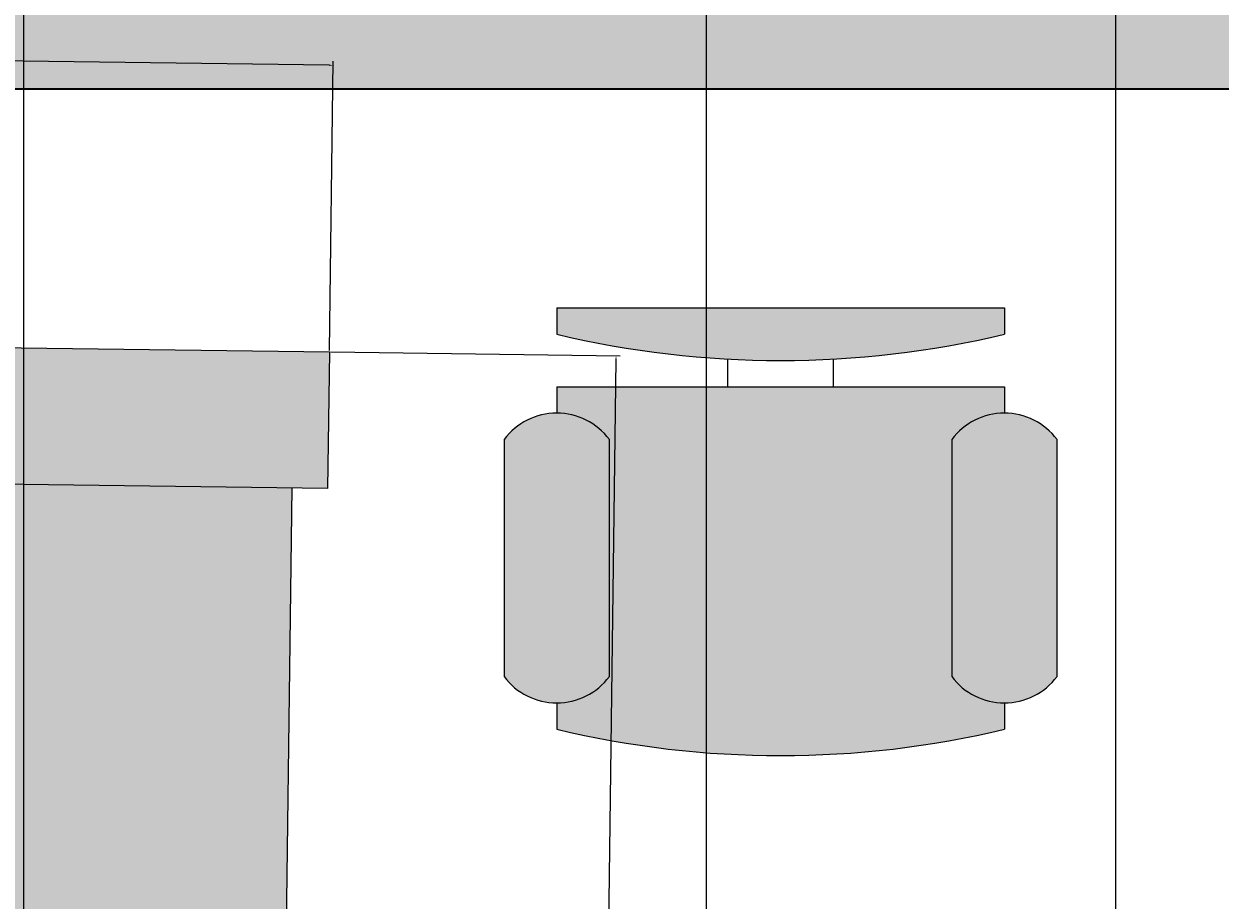
# Model space of a CAD drawing. Units: inches. Extents: x 1567 to 1964, y 1813 to 2447.
# Tile 10 of 28: x 1630 to 1683, y 2224 to 2262. Entities that reach past the tile are written whole.
import ezdxf

# ---------------------------------------------------------------- set-up
doc = ezdxf.new("R2010")
doc.units = ezdxf.units.IN
for name, color, linetype, lineweight in [('A-ANNO-DIMS', 2, 'Continuous', 18), ('A-FURN', 8, 'Continuous', 18), ('A-WALL', 7, 'Continuous', 35)]:
    doc.layers.add(name, color=color, linetype=linetype, lineweight=lineweight)
doc.layers.add('A-FURN-PATT', color=252, linetype='Continuous', lineweight=13, true_color=0x939598)
doc.layers.add('A-WALL-PATT', color=251, linetype='Continuous', lineweight=13, true_color=0x636466)
doc.styles.get("Standard").update_dxf_attribs({"font": 'arial.ttf'})
doc.dimstyles.get("Standard").update_dxf_attribs({"dimtxt": 0.18, "dimasz": 0.18, "dimexe": 0.18, "dimexo": 0.0625, "dimgap": 0.09, "dimtad": 0, "dimtih": 1, "dimtoh": 1, "dimdec": 4, "dimzin": 0, "dimdsep": 46, "dimtxsty": 'Standard', "dimcen": 0.09, "dimadec": 0, "dimazin": 0, "dimtfac": 1, "dimtdec": 4, "dimtofl": 0, "dimtmove": 0, "dimatfit": 3, "dimfxl": 1, "dimtolj": 1, "dimtzin": 0, "dimarcsym": 0})

# ---------------------------------------------------------------- blocks, each defined once
blk = doc.blocks.new('Sofa - Roundback 7 ft.')
for p, q in [((35.99998, -34), (35.99998, -11.4696)), ((-36.000027, -32.4421), (35.99998, -32.4421))]:
    blk.add_line(p, q)
blk.add_lwpolyline([(41.99998, -8), (41.99998, -34), (35.99998, -34)])
blk = doc.blocks.new('Chair - Desk')
for p, q in [((-8.5, 0), (-8.5, -1)), ((-8.5, 0), (8.5, 0)), ((8.5, 0), (8.5, -1)), ((-2, -3), (-2, -1.9355)), ((2, -1.9576), (2, -3)), ((-8.5, -3), (-8.5, -4)), ((-8.5, -3), (8.5, -3)), ((8.5, -3), (8.5, -4)), ((-10.5, -5), (-10.5, -14)), ((-6.5, -14), (-6.5, -5)), ((6.5, -5), (6.5, -14)), ((10.5, -14), (10.5, -5)), ((-8.5, -15), (-8.5, -16)), ((8.5, -15), (8.5, -16))]:
    blk.add_line(p, q)
for centre, radius, start, end in [((0, 34.625), 36.625, 256.5803, 283.4197), ((-8.5, -6.5), 2.5, 36.8699, 143.1301), ((8.5, -6.5), 2.5, 36.8699, 143.1301), ((-8.5, -12.5), 2.5, 216.8699, 323.1301), ((8.5, -12.5), 2.5, 216.8699, 323.1301), ((0, 19.625), 36.625, 256.5803, 283.4197)]:
    blk.add_arc(centre, radius, start, end)
blk = doc.blocks.new('*D23')
at = {"layer": 'A-ANNO-DIMS', "color": 0, "lineweight": -2, "transparency": 16777216}
for p, q in [((1643.923, 2247.723), (1656.64, 2247.554)), ((1656.457, 2247.376), (1655.905, 2205.743)), ((1655.347, 2163.744), (1655.9, 2205.377)), ((1642.808, 2163.73), (1655.525, 2163.561))]:
    blk.add_line(p, q, dxfattribs=at)
at = {"layer": 'A-ANNO-DIMS', "color": 0, "transparency": 16777216}
for points in [[(1656.427, 2247.377), (1656.487, 2247.376), (1656.46, 2247.556)], [(1655.317, 2163.744), (1655.377, 2163.743), (1655.345, 2163.564)]]:
    blk.add_solid(points, dxfattribs=at)
at = {"layer": 'Defpoints', "color": 0, "transparency": 16777216}
for p in [(1643.861, 2247.723), (1656.46, 2247.556), (1642.746, 2163.731)]:
    blk.add_point(p, dxfattribs=at)
at = {"layer": 'A-ANNO-DIMS', "color": 0, "transparency": 16777216, "insert": (1655.902, 2205.56), "char_height": 0.18, "attachment_point": 5}
blk.add_mtext('\\A1;SOFA 84', dxfattribs=at)
blk = doc.blocks.new('*D24')
at = {"layer": 'A-ANNO-DIMS', "color": 0, "lineweight": -2, "transparency": 16777216}
for p, q in [((1607.198, 2248.273), (1607.367, 2260.989)), ((1607.544, 2260.807), (1625.477, 2260.569)), ((1643.848, 2260.325), (1625.915, 2260.563)), ((1643.862, 2247.786), (1644.03, 2260.502))]:
    blk.add_line(p, q, dxfattribs=at)
at = {"layer": 'A-ANNO-DIMS', "color": 0, "transparency": 16777216}
for points in [[(1607.545, 2260.837), (1607.544, 2260.777), (1607.364, 2260.809)], [(1643.848, 2260.355), (1643.848, 2260.295), (1644.028, 2260.322)]]:
    blk.add_solid(points, dxfattribs=at)
at = {"layer": 'Defpoints', "color": 0, "transparency": 16777216}
for p in [(1607.364, 2260.809), (1607.197, 2248.21), (1643.861, 2247.723)]:
    blk.add_point(p, dxfattribs=at)
at = {"layer": 'A-ANNO-DIMS', "color": 0, "transparency": 16777216, "insert": (1625.696, 2260.566), "char_height": 0.18, "attachment_point": 5}
blk.add_mtext('\\A1;37', dxfattribs=at)
blk = doc.blocks.new('*D57')
at = {"layer": 'A-ANNO-DIMS', "color": 0, "lineweight": -2, "transparency": 16777216}
for p, q in [((1630.43, 2127.352), (1630.43, 2447.12)), ((1630.61, 2446.94), (1654.207, 2446.94)), ((1678.25, 2446.94), (1654.652, 2446.94)), ((1678.43, 2127.352), (1678.43, 2447.12))]:
    blk.add_line(p, q, dxfattribs=at)
at = {"layer": 'A-ANNO-DIMS', "color": 0, "transparency": 16777216}
for points in [[(1630.61, 2446.97), (1630.61, 2446.91), (1630.43, 2446.94)], [(1678.25, 2446.97), (1678.25, 2446.91), (1678.43, 2446.94)]]:
    blk.add_solid(points, dxfattribs=at)
at = {"layer": 'Defpoints', "color": 0, "transparency": 16777216}
for p in [(1678.43, 2446.94), (1630.43, 2127.29), (1678.43, 2127.29)]:
    blk.add_point(p, dxfattribs=at)
at = {"layer": 'A-ANNO-DIMS', "color": 0, "transparency": 16777216, "insert": (1654.43, 2446.94), "char_height": 0.18, "attachment_point": 5}
blk.add_mtext('\\A1;48', dxfattribs=at)
blk = doc.blocks.new('*D60')
at = {"layer": 'A-ANNO-DIMS', "color": 0, "lineweight": -2, "transparency": 16777216}
for p, q in [((1660.43, 2063.352), (1660.43, 2447.12)), ((1660.61, 2446.94), (1681.208, 2446.94)), ((1702.25, 2446.94), (1681.651, 2446.94)), ((1702.43, 2063.352), (1702.43, 2447.12))]:
    blk.add_line(p, q, dxfattribs=at)
at = {"layer": 'A-ANNO-DIMS', "color": 0, "transparency": 16777216}
for points in [[(1660.61, 2446.97), (1660.61, 2446.91), (1660.43, 2446.94)], [(1702.25, 2446.97), (1702.25, 2446.91), (1702.43, 2446.94)]]:
    blk.add_solid(points, dxfattribs=at)
at = {"layer": 'Defpoints', "color": 0, "transparency": 16777216}
for p in [(1660.43, 2446.94), (1660.43, 2063.29), (1702.43, 2063.29)]:
    blk.add_point(p, dxfattribs=at)
at = {"layer": 'A-ANNO-DIMS', "color": 0, "transparency": 16777216, "insert": (1681.43, 2446.94), "char_height": 0.18, "attachment_point": 5}
blk.add_mtext('\\A1;42', dxfattribs=at)

msp = doc.modelspace()

# ---------------------------------------------------------------- hatches: boundary and pattern name
at = {"layer": 'A-FURN-PATT'}
h = msp.add_hatch(color=256, dxfattribs=at)
h.dxf.hatch_style = 1
h.paths.add_polyline_path([(1621.2532, 2242.0229), (1643.7811, 2241.7239), (1643.8607, 2247.7234), (1617.863, 2248.0685, 0.1904762), (1616.7481, 2164.0759), (1642.7458, 2163.7308), (1642.8254, 2169.7302), (1620.2975, 2170.0293, -0.1519478)])
h.paths.add_polyline_path([(1673.5306, 2249.6607), (1653.8509, 2249.6607), (1653.8509, 2248.5031, 0.1176471), (1673.5306, 2248.5031)])
h.paths.add_polyline_path([(1706.0889, 2249.6607), (1686.4092, 2249.6607), (1686.4092, 2248.5031, 0.1176471), (1706.0889, 2248.5031)])
h.paths.add_polyline_path([(1782.4511, 2227.4197), (1766.4511, 2227.4197), (1766.2949, 2226.4197), (1782.6074, 2226.4197)])
h.paths.add_polyline_path([(1810.4511, 2227.4197), (1794.4511, 2227.4197), (1794.2949, 2226.4197), (1810.6074, 2226.4197)])
h.paths.add_polyline_path([(1743.9511, 2208.076), (1742.9511, 2207.9197), (1742.9511, 2191.9197), (1743.9511, 2191.7635)])
h.paths.add_polyline_path([(1782.6074, 2173.4197), (1766.2949, 2173.4197), (1766.4511, 2172.4197), (1782.4511, 2172.4197)])
h.paths.add_polyline_path([(1810.6074, 2173.4197), (1794.2949, 2173.4197), (1794.4511, 2172.4197), (1810.4511, 2172.4197)])
h.paths.add_polyline_path([(1861.053, 2006.5071), (1845.8531, 2006.5071), (1861.053, 1991.3071)])
h.paths.add_polyline_path([(1905.853, 1993.7071), (1861.053, 1993.7071), (1861.053, 1991.3071), (1905.853, 1991.3071)])
h.paths.add_polyline_path([(1919.7245, 2257.29, 0.5000001), (1918.7245, 2258.29), (1901.7245, 2258.29, 0.5000001), (1900.7245, 2257.29), (1900.7245, 2253.29, 0.5000001), (1901.7245, 2252.29), (1918.7245, 2252.29, 0.5000001), (1919.7245, 2253.29)])
h.paths.add_polyline_path([(1875.9094, 2391.0204), (1875.9094, 2375.8204), (1891.1093, 2375.8204)], flags=17)
h.paths.add_polyline_path([(1891.1093, 2405.4204), (1831.1094, 2405.4204), (1831.1094, 2391.0204), (1839.1093, 2391.0204), (1839.1093, 2404.2204), (1859.9093, 2404.2204), (1859.9093, 2391.0204), (1862.3093, 2391.0204), (1862.3093, 2404.2204), (1883.1093, 2404.2204), (1883.1093, 2389.0204), (1877.9094, 2389.0204), (1891.1093, 2375.8204)])
h.paths.add_polyline_path([(1682.1402, 2390.0316), (1682.1402, 2374.8316), (1697.3402, 2374.8316)], flags=17)
h.paths.add_polyline_path([(1697.3402, 2404.4316), (1637.3402, 2404.4316), (1637.3402, 2390.0316), (1645.3402, 2390.0316), (1645.3402, 2403.2316), (1666.1402, 2403.2316), (1666.1402, 2390.0316), (1668.5402, 2390.0316), (1668.5402, 2403.2316), (1689.3402, 2403.2316), (1689.3402, 2388.0316), (1684.1402, 2388.0316), (1697.3402, 2374.8316)])
h = msp.add_hatch(color=256, dxfattribs=at)
h.dxf.hatch_style = 1
h.paths.add_polyline_path([(1642.2233, 2241.7446), (1623.1648, 2241.9976), (1622.8462, 2217.9997), (1641.9047, 2217.7467)])
h.paths.add_polyline_path([(1641.9047, 2217.7467), (1622.8462, 2217.9997), (1622.5277, 2194.0018), (1641.5862, 2193.7488)])
h.paths.add_polyline_path([(1641.5862, 2193.7488), (1622.5277, 2194.0018), (1622.2091, 2170.0039), (1641.2677, 2169.7509)])
h.paths.add_polyline_path([(1671.2154, 2243.8726, -0.236068), (1673.5306, 2245.0302), (1673.5306, 2246.1879), (1653.8509, 2246.1879), (1653.8509, 2245.0302, -0.236068), (1656.1662, 2243.8726), (1656.1662, 2233.4539, -0.236068), (1653.8509, 2232.2963), (1653.8509, 2231.1387, 0.1176471), (1673.5306, 2231.1387), (1673.5306, 2232.2963, -0.236068), (1671.2154, 2233.4539)])
h.paths.add_polyline_path([(1703.7736, 2243.8726, -0.236068), (1706.0889, 2245.0302), (1706.0889, 2246.1879), (1686.4092, 2246.1879), (1686.4092, 2245.0302, -0.236068), (1688.7245, 2243.8726), (1688.7245, 2233.4539, -0.236068), (1686.4092, 2232.2963), (1686.4092, 2231.1387, 0.1176471), (1706.0889, 2231.1387), (1706.0889, 2232.2963, -0.236068), (1703.7736, 2233.4539)])
h.paths.add_polyline_path([(1782.6855, 2225.9197), (1766.2168, 2225.9197), (1764.9668, 2217.9197), (1783.9356, 2217.9197)])
h.paths.add_polyline_path([(1810.6855, 2225.9197), (1794.2168, 2225.9197), (1792.9668, 2217.9197), (1811.9356, 2217.9197)])
h.paths.add_polyline_path([(1752.4511, 2209.4041), (1744.4511, 2208.1541), (1744.4511, 2191.6853), (1752.4511, 2190.4354)])
h.paths.add_polyline_path([(1783.9356, 2181.9197), (1764.9668, 2181.9197), (1766.2168, 2173.9197), (1782.6855, 2173.9197)])
h.paths.add_polyline_path([(1811.9356, 2181.9197), (1792.9668, 2181.9197), (1794.2168, 2173.9197), (1810.6855, 2173.9197)])
h.paths.add_polyline_path([(1832.4511, 2208.1541), (1824.4511, 2209.4041), (1824.4511, 2190.4354), (1832.4511, 2191.6853)])
h.paths.add_polyline_path([(1824.4511, 2194.4197), (1823.8775, 2194.266), (1823.2838, 2194.1743), (1822.6735, 2194.1363), (1822.0501, 2194.1437), (1821.4169, 2194.1882), (1820.7773, 2194.2615), (1820.1348, 2194.3554), (1819.4928, 2194.4614), (1818.8527, 2194.5726), (1818.2083, 2194.6873), (1817.5511, 2194.8049), (1816.873, 2194.9249), (1816.1656, 2195.0469), (1815.4205, 2195.1704), (1814.6296, 2195.2948), (1813.7845, 2195.4197), (1812.88, 2195.5442), (1811.9238, 2195.6658), (1810.9265, 2195.7815), (1809.899, 2195.8885), (1808.852, 2195.9837), (1807.7962, 2196.0643), (1806.7423, 2196.1273), (1805.7011, 2196.1697), (1804.6806, 2196.1896), (1803.6777, 2196.188), (1802.6865, 2196.1668), (1801.7011, 2196.1281), (1800.7158, 2196.0737), (1799.7245, 2196.0057), (1798.7216, 2195.9259), (1797.7011, 2195.8364), (1796.6564, 2195.7387), (1795.5781, 2195.6333), (1794.4557, 2195.52), (1793.2792, 2195.3989), (1792.0383, 2195.27), (1790.7226, 2195.1333), (1789.3219, 2194.9887), (1787.8261, 2194.8364), (1786.1882, 2194.6764), (1784.2148, 2194.5096), (1781.6759, 2194.3369), (1778.3417, 2194.1593), (1773.9821, 2193.9778), (1768.3671, 2193.7934), (1761.2668, 2193.6071), (1752.4511, 2193.4197), (1752.4511, 2189.9197), (1762.0489, 2190.1067), (1769.9836, 2190.2908), (1776.4672, 2190.469), (1781.7115, 2190.6385), (1785.9285, 2190.7962), (1789.33, 2190.9393), (1792.128, 2191.0648), (1794.5344, 2191.1697), (1796.7278, 2191.2521), (1798.7532, 2191.313), (1800.6223, 2191.3543), (1802.3469, 2191.3781), (1803.9387, 2191.3862), (1805.4094, 2191.3807), (1806.7708, 2191.3634), (1808.0345, 2191.3364), (1809.2127, 2191.3013), (1810.3196, 2191.2589), (1811.3699, 2191.2097), (1812.3782, 2191.1541), (1813.3592, 2191.0927), (1814.3274, 2191.0259), (1815.2976, 2190.9542), (1816.2845, 2190.8781), (1817.2985, 2190.7986), (1818.3339, 2190.7186), (1819.3811, 2190.6415), (1820.4303, 2190.5708), (1821.4716, 2190.5098), (1822.4954, 2190.4621), (1823.4918, 2190.4309), (1824.3581, 2190.4208), (1824.4511, 2190.4354)])
h.paths.add_polyline_path([(1874.6531, 1991.3071), (1861.053, 1991.3071), (1859.053, 1993.3071), (1853.8531, 1993.3071), (1853.8531, 1978.1071), (1874.6531, 1978.1071)], flags=17)
h.paths.add_polyline_path([(1897.8531, 1991.3071), (1877.0531, 1991.3071), (1877.0531, 1978.1071), (1897.8531, 1978.1071)], flags=17)
h.paths.add_polyline_path([(1853.8531, 1993.3071), (1859.053, 1993.3071), (1845.8531, 2006.5071), (1845.8531, 1976.9071), (1905.853, 1976.9071), (1905.853, 1991.3071), (1897.8531, 1991.3071), (1897.8531, 1978.1071), (1877.0531, 1978.1071), (1877.0531, 1991.3071), (1874.6531, 1991.3071), (1874.6531, 1978.1071), (1853.8531, 1978.1071)])
h.paths.add_polyline_path([(1920.7245, 2259.29), (1899.7245, 2259.29), (1899.7245, 2251.29), (1920.7245, 2251.29)])
h.paths.add_polyline_path([(1918.7245, 2252.29, 0.5000001), (1919.7245, 2253.29), (1919.7245, 2257.29, 0.5000001), (1918.7245, 2258.29), (1901.7245, 2258.29, 0.5000001), (1900.7245, 2257.29), (1900.7245, 2253.29, 0.5000001), (1901.7245, 2252.29)], flags=16)
h.paths.add_polyline_path([(1843.2327, 2065.967), (1919.26, 2065.967), (1919.26, 2095.8187), (1843.2327, 2095.8187)], flags=9)
h = msp.add_hatch(color=256, dxfattribs=at)
h.dxf.hatch_style = 1
h.paths.add_polyline_path([(1622.8462, 2217.9997), (1616.0605, 2218.0897, 0.0496282), (1615.7419, 2194.0919), (1622.5277, 2194.0018)])
h.paths.add_polyline_path([(1623.1648, 2241.9976), (1621.2532, 2242.0229, 0.0506467), (1616.0605, 2218.0897), (1622.8462, 2217.9997)])
h.paths.add_polyline_path([(1622.5277, 2194.0018), (1615.7419, 2194.0919, 0.0506466), (1620.2975, 2170.0293), (1622.2091, 2170.0039)])
h.paths.add_polyline_path([(1656.1662, 2243.8726, 0.5), (1651.5357, 2243.8726), (1651.5357, 2233.4539, 0.5), (1656.1662, 2233.4539)])
h.paths.add_polyline_path([(1675.8459, 2243.8726, 0.5), (1671.2154, 2243.8726), (1671.2154, 2233.4539, 0.5), (1675.8459, 2233.4539)])
h.paths.add_polyline_path([(1688.7245, 2243.8726, 0.5), (1684.094, 2243.8726), (1684.094, 2233.4539, 0.5), (1688.7245, 2233.4539)])
h.paths.add_polyline_path([(1708.4042, 2243.8726, 0.5), (1703.7736, 2243.8726), (1703.7736, 2233.4539, 0.5), (1708.4042, 2233.4539)])
at = {"layer": 'A-WALL-PATT'}
h = msp.add_hatch(color=256, dxfattribs=at)
h.dxf.hatch_style = 1
h.paths.add_polyline_path([(1606.4295, 2407.29), (1654.4295, 2407.29), (1654.4295, 2416.29), (1597.4295, 2416.29), (1597.4295, 2217.29), (1606.4295, 2217.29), (1606.4295, 2259.29), (1738.4295, 2259.29), (1738.4295, 2247.29), (1742.4295, 2247.29), (1742.4295, 2259.29), (1742.4295, 2272.29), (1738.4295, 2272.29), (1738.4295, 2263.29), (1606.4295, 2263.29)])
h.paths.add_polyline_path([(1753.4295, 2416.29), (1690.4295, 2416.29), (1690.4295, 2407.29), (1738.4295, 2407.29), (1738.4295, 2308.29), (1742.4295, 2308.29), (1742.4295, 2331.29), (1746.9295, 2331.29), (1746.9295, 2335.29), (1742.4295, 2335.29), (1742.4295, 2407.29), (1753.4295, 2407.29)])
h.paths.add_polyline_path([(1840.4295, 2416.29), (1777.4295, 2416.29), (1777.4295, 2407.29), (1788.4295, 2407.29), (1788.4295, 2335.29), (1776.9295, 2335.29), (1776.9295, 2331.29), (1788.4295, 2331.29), (1788.4295, 2308.29), (1792.4295, 2308.29), (1792.4295, 2407.29), (1840.4295, 2407.29)])
h.paths.add_polyline_path([(1933.4295, 2416.29), (1876.4295, 2416.29), (1876.4295, 2407.29), (1924.4295, 2407.29), (1924.4295, 2263.29), (1792.4295, 2263.29), (1792.4295, 2272.29), (1788.4295, 2272.29), (1788.4295, 2259.29), (1872.4295, 2259.29), (1872.4295, 2171.29), (1880.9295, 2171.29), (1880.9295, 2175.29), (1876.4295, 2175.29), (1876.4295, 2259.29), (1924.4295, 2259.29), (1924.4295, 2229.29), (1933.4295, 2229.29)])
h.paths.add_polyline_path([(1933.4295, 2205.29), (1924.4295, 2205.29), (1924.4295, 2175.29), (1910.9295, 2175.29), (1910.9295, 2171.29), (1924.4295, 2171.29), (1924.4295, 2127.29), (1844.4295, 2127.29), (1844.4295, 2123.29), (1924.4295, 2123.29), (1924.4295, 2063.29), (1933.4295, 2063.29)])
h.paths.add_polyline_path([(1799.4295, 2123.29), (1808.4295, 2123.29), (1808.4295, 2127.29), (1781.4295, 2127.29), (1781.4295, 2123.29), (1795.4295, 2123.29), (1795.4295, 1964.29), (1711.4295, 1964.29), (1711.4295, 2123.29), (1751.4295, 2123.29), (1751.4295, 2127.29), (1742.4295, 2127.29), (1742.4295, 2139.29), (1738.4295, 2139.29), (1738.4295, 2127.29), (1678.4295, 2127.29), (1678.4295, 2123.29), (1702.4295, 2123.29), (1702.4295, 1913.29), (1678.4295, 1913.29), (1678.4295, 1904.29), (1711.4295, 1904.29), (1711.4295, 1960.29), (1795.4295, 1960.29), (1795.4295, 1906.69), (1929.4295, 1906.69), (1929.4295, 1848.29), (1601.4295, 1848.29), (1601.4295, 1904.29), (1630.4295, 1904.29), (1630.4295, 1913.29), (1606.4295, 1913.29), (1606.4295, 2123.29), (1630.4295, 2123.29), (1630.4295, 2127.29), (1606.4295, 2127.29), (1606.4295, 2169.29), (1597.4295, 2169.29), (1597.4295, 1844.29), (1933.4295, 1844.29), (1933.4295, 2027.29), (1924.4295, 2027.29), (1924.4295, 1967.29), (1833.9295, 1967.29), (1833.9295, 1963.29), (1924.4295, 1963.29), (1924.4295, 1910.69), (1799.4295, 1910.69), (1799.4295, 1963.29), (1803.9295, 1963.29), (1803.9295, 1967.29), (1799.4295, 1967.29)])

# ---------------------------------------------------------------- linework, layer by layer
at = {"layer": 'A-WALL'}
msp.add_line((1606.4295, 2259.29), (1738.4295, 2259.29), dxfattribs=at)

# ---------------------------------------------------------------- block references
at = {"layer": 'A-FURN', "xscale": 1.157629009682769, "yscale": 1.157629009682769, "zscale": 1.157629009682769}
msp.add_blockref('Chair - Desk', (1663.6908, 2249.6607), dxfattribs=at)
at = {"layer": 'A-FURN', "rotation": 89.2395118843373}
msp.add_blockref('Sofa - Roundback 7 ft.', (1609.3062, 2206.1784), dxfattribs=at)

# ---------------------------------------------------------------- dimensions: what is measured, and where the dimension line sits
at = {"layer": 'A-ANNO-DIMS'}
for base, p1, p2, picture, middle in [((1678.4295, 2446.94), (1630.4295, 2127.29), (1678.4295, 2127.29), '*D57', (1654.4295, 2446.94)), ((1660.4295, 2446.94), (1702.4295, 2063.29), (1660.4295, 2063.29), '*D60', (1681.4295, 2446.94))]:
    dim = msp.add_linear_dim(base=base, p1=p1, p2=p2, dimstyle='Standard', override={"dimdec": 0, "dimlfac": 1, "dimrnd": 0, "dimzin": 0, "dimdsep": 46, "dimlunit": 2}, dxfattribs=at)
    dim.commit()
    dim.dimension.update_dxf_attribs({"geometry": picture, "text_midpoint": middle})
dim = msp.add_linear_dim(base=(1607.3645, 2260.8089), p1=(1643.8607, 2247.7234), p2=(1607.1972, 2248.21), angle=179.23951, dimstyle='Standard', override={"dimdec": 0, "dimlfac": 1, "dimrnd": 0, "dimzin": 0, "dimdsep": 46, "dimlunit": 2}, dxfattribs=at)
dim.commit()
dim.dimension.update_dxf_attribs({"geometry": '*D24', "text_midpoint": (1625.6962, 2260.5656)})
dim = msp.add_linear_dim(base=(1656.4596, 2247.5562), p1=(1642.7458, 2163.7308), p2=(1643.8607, 2247.7234), angle=89.23951, text='SOFA <>', dimstyle='Standard', override={"dimdec": 0, "dimlfac": 1, "dimrnd": 0, "dimzin": 0, "dimdsep": 46, "dimlunit": 2}, dxfattribs=at)
dim.commit()
dim.dimension.update_dxf_attribs({"geometry": '*D23', "text_midpoint": (1655.9021, 2205.5598)})

doc.saveas('drawing.dxf')
